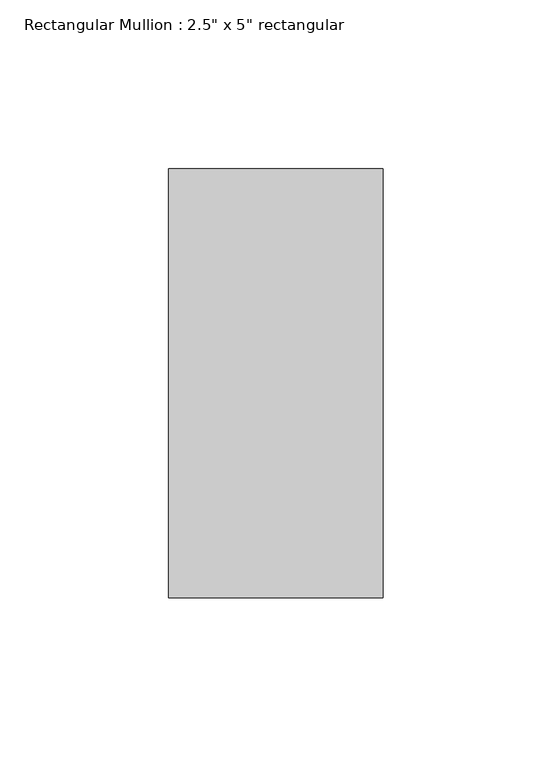
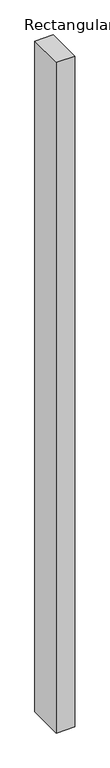
"""IFC4 building model written with IfcOpenShell, lengths in millimetres: member geometry."""

from ifc_helpers import new_model, si_unit, frame, origin, place, context, project, spatial, polyline, outline, extrude, source, transform, mapped, element, save


def member_40a3ee5d(model_context):
    return source(origin(), model_context, "Body", "SweptSolid", [
        extrude(outline(polyline([(0.0, 63.5), (0.0, -63.5), (-63.5, -63.5), (-63.5, 63.5), (0.0, 63.5)])), frame((0.0, 0.0, -2440.0217298), z_axis=(0.0, 0.0, 1.0), x_axis=(1.0, 0.0, 0.0)), (0.0, 0.0, 1.0), 2440.0217298),
    ])


if __name__ == "__main__":
    model = new_model("IFC4")
    model_context = context("Model", 3, world=origin())
    ifc_project = project(units=[si_unit("LENGTHUNIT", "METRE", prefix="MILLI")], contexts=[model_context])
    site = spatial("IfcSite", under=ifc_project)
    building = spatial("IfcBuilding", under=site)
    placement = place(None, origin())
    member_shape = member_40a3ee5d(model_context)
    element("IfcMember", 1, ObjectType="Rectangular Mullion : 2.5\" x 5\" rectangular", at=placement, inside=building, context=model_context, shape_type="MappedRepresentation", body=[
        mapped(member_shape, transform((0.0, 0.0, 0.0), x_axis=(1.0, 0.0, 0.0), y_axis=(0.0, 1.0, 0.0), z_axis=(0.0, 0.0, 1.0))),
    ])
    save(model, "model.ifc")

# Revit data of these elements
# Type "Rectangular Mullion : 2.5\" x 5\" rectangular"
#   built-in parameter 1007304 = 0.416667 (stored number, unit not read)
#   built-in parameter 1007301 = 0.104167 (stored number, unit not read)
#   built-in parameter 1007300 = 0.104167 (stored number, unit not read)
# Element 1 (IfcMember, "Rectangular Mullion : 2.5\" x 5\" rectangular")
#   Materials on its faces: "Aluminum"
# Materials
#   "Aluminum": class "Metal", colour RGB 247 247 247, transparency 0, Description = "Aluminum 6061", Cost = 0
